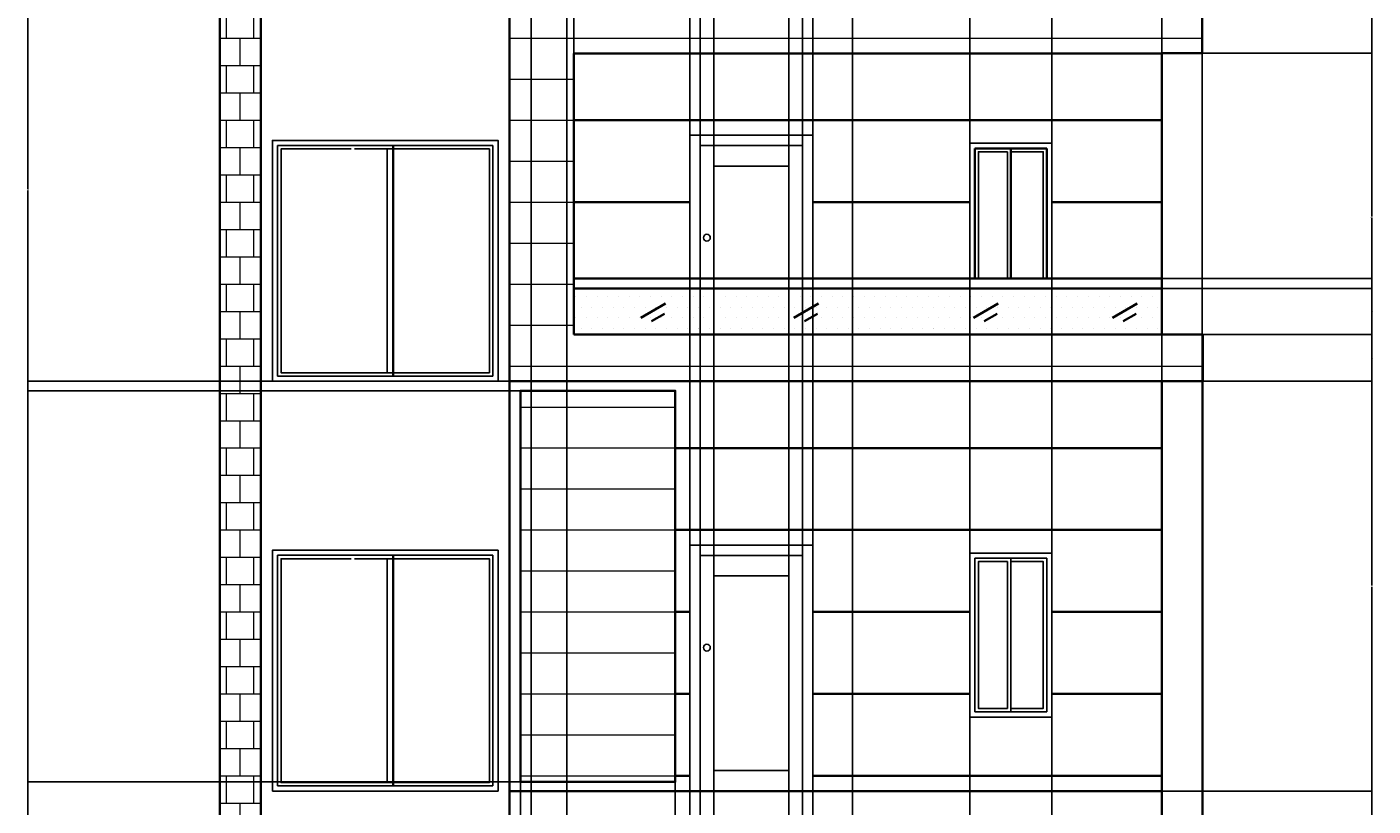
# Model space of a CAD drawing. Units: inches. Extents: x 10 to 404, y -77 to 696.
# Tile 3 of 5: x 10 to 404, y 135 to 363. Entities that reach past the tile are written whole.
import ezdxf

# ---------------------------------------------------------------- set-up
doc = ezdxf.new("R2010")
doc.units = ezdxf.units.IN
doc.header["$MEASUREMENT"] = 0
for name, color, linetype, lineweight in [('A-ANNO-DIMS', 2, 'Continuous', 18), ('A-DOOR', 4, 'Continuous', 25), ('A-ELEV', 7, 'Continuous', 35), ('A-ELEV-PATT', 8, 'Continuous', 13), ('A-GLAZ', 4, 'Continuous', 25)]:
    doc.layers.add(name, color=color, linetype=linetype, lineweight=lineweight)
doc.styles.get("Standard").update_dxf_attribs({"font": 'arial.ttf'})
doc.dimstyles.get("Standard").update_dxf_attribs({"dimtxt": 0.18, "dimasz": 0.18, "dimexe": 0.18, "dimexo": 0.0625, "dimgap": 0.09, "dimtad": 0, "dimtih": 1, "dimtoh": 1, "dimdec": 4, "dimzin": 0, "dimdsep": 46, "dimtxsty": 'Standard', "dimcen": 0.09, "dimadec": 0, "dimazin": 0, "dimtfac": 1, "dimtdec": 4, "dimtofl": 0, "dimtmove": 0, "dimatfit": 3, "dimfxl": 1, "dimtolj": 1, "dimtzin": 0, "dimarcsym": 0})

# ---------------------------------------------------------------- blocks, each defined once
blk = doc.blocks.new('*U5')
for p, q in [((1.5, 1.5), (1.5, 46.5)), ((1.5, 46.5), (12, 46.5)), ((12, 1.5), (12, 46.5)), ((12, 46.5), (22.5, 46.5)), ((22.5, 46.5), (22.5, 1.5)), ((12, 1.5), (1.5, 1.5)), ((22.5, 1.5), (12, 1.5))]:
    blk.add_line(p, q)
blk.add_lwpolyline([(0, 0), (0, 48), (24, 48), (24, 0)], close=True)
for points in [[(11, 45.5), (11, 2.5), (2.5, 2.5), (2.5, 45.5), (11, 45.5)], [(12, 45.5), (21.5, 45.5), (21.5, 2.5), (12, 2.5)]]:
    blk.add_lwpolyline(points)
blk = doc.blocks.new('*U4')
blk.add_lwpolyline([(3.12, 0.01), (0.12, 0.01), (0.12, 72.01), (36.12, 72.01), (36.12, 0.01), (33.12, 0.01)])
for points in [[(33.12, 68.99), (33.12, 0.01), (3.12, 0.01), (3.12, 68.99)], [(29.12, 6.01), (29.12, 62.99), (7.12, 62.99), (7.12, 6.01)]]:
    blk.add_lwpolyline(points, close=True)
blk.add_circle((31.12, 42.01), 1)
blk = doc.blocks.new('WIN-SLIDING-2P')
for p, q in [((83.01, 21.05), (83.01, 88.58)), ((83.01, 88.58), (105.51, 88.58)), ((105.51, 88.58), (146.03, 88.58)), ((146.03, 88.58), (146.03, 21.05)), ((105.51, 21.05), (83.01, 21.05)), ((146.03, 21.05), (105.51, 21.05))]:
    blk.add_line(p, q)
blk.add_lwpolyline([(81.51, 19.55), (81.51, 90.08), (147.53, 90.08), (147.53, 19.55)], close=True)
blk.add_lwpolyline([(115.07, 87.58), (115.07, 22.05), (84.01, 22.05), (84.01, 87.58), (104.51, 87.58)])
blk = doc.blocks.new('*D10')
at = {"layer": 'A-ANNO-DIMS', "color": 0, "lineweight": -2, "transparency": 16777216}
for p, q in [((65.94, 657.96), (9.76, 657.96)), ((9.94, 657.78), (9.94, 315.77)), ((9.94, -26.6), (9.94, 315.41)), ((176.46, -26.78), (9.76, -26.78))]:
    blk.add_line(p, q, dxfattribs=at)
at = {"layer": 'A-ANNO-DIMS', "color": 0, "transparency": 16777216}
for points in [[(9.91, 657.78), (9.97, 657.78), (9.94, 657.96)], [(9.91, -26.6), (9.97, -26.6), (9.94, -26.78)]]:
    blk.add_solid(points, dxfattribs=at)
at = {"layer": 'Defpoints', "color": 0, "transparency": 16777216}
for p in [(9.94, 657.96), (66.01, 657.96), (176.53, -26.78)]:
    blk.add_point(p, dxfattribs=at)
at = {"layer": 'A-ANNO-DIMS', "color": 0, "transparency": 16777216, "insert": (9.94, 315.59), "char_height": 0.18, "attachment_point": 5}
blk.add_mtext('\\A1;684.7', dxfattribs=at)
blk = doc.blocks.new('*D23')
at = {"layer": 'A-ANNO-DIMS', "color": 0, "lineweight": -2, "transparency": 16777216}
for p, q in [((341.87, 355.52), (341.87, -64.31)), ((353.59, 355.52), (353.59, -64.31)), ((342.05, -64.13), (347.27, -64.13)), ((353.41, -64.13), (348.18, -64.13))]:
    blk.add_line(p, q, dxfattribs=at)
at = {"layer": 'A-ANNO-DIMS', "color": 0, "transparency": 16777216}
for points in [[(342.05, -64.1), (342.05, -64.16), (341.87, -64.13)], [(353.41, -64.1), (353.41, -64.16), (353.59, -64.13)]]:
    blk.add_solid(points, dxfattribs=at)
at = {"layer": 'Defpoints', "color": 0, "transparency": 16777216}
for p in [(341.87, 355.58), (353.59, 355.58), (353.59, -64.13)]:
    blk.add_point(p, dxfattribs=at)
at = {"layer": 'A-ANNO-DIMS', "color": 0, "transparency": 16777216, "insert": (347.73, -64.13), "char_height": 0.18, "attachment_point": 5}
blk.add_mtext('\\A1;11.723', dxfattribs=at)
blk = doc.blocks.new('*D28')
at = {"layer": 'A-ANNO-DIMS', "color": 0, "lineweight": -2, "transparency": 16777216}
for p, q in [((341.93, 139.55), (403.47, 139.55)), ((403.29, 139.37), (403.29, 79.74)), ((403.29, 19.73), (403.29, 79.37)), ((341.93, 19.55), (403.47, 19.55))]:
    blk.add_line(p, q, dxfattribs=at)
at = {"layer": 'A-ANNO-DIMS', "color": 0, "transparency": 16777216}
for points in [[(403.26, 139.37), (403.32, 139.37), (403.29, 139.55)], [(403.26, 19.73), (403.32, 19.73), (403.29, 19.55)]]:
    blk.add_solid(points, dxfattribs=at)
at = {"layer": 'Defpoints', "color": 0, "transparency": 16777216}
for p in [(341.87, 139.55), (403.29, 139.55), (341.87, 19.55)]:
    blk.add_point(p, dxfattribs=at)
at = {"layer": 'A-ANNO-DIMS', "color": 0, "transparency": 16777216, "insert": (403.29, 79.55), "char_height": 0.18, "attachment_point": 5}
blk.add_mtext('\\A1;120', dxfattribs=at)
blk = doc.blocks.new('*D29')
at = {"layer": 'A-ANNO-DIMS', "color": 0, "lineweight": -2, "transparency": 16777216}
for p, q in [((341.93, 259.55), (403.47, 259.55)), ((403.29, 259.37), (403.29, 199.74)), ((403.29, 139.73), (403.29, 199.37)), ((341.93, 139.55), (403.47, 139.55))]:
    blk.add_line(p, q, dxfattribs=at)
at = {"layer": 'A-ANNO-DIMS', "color": 0, "transparency": 16777216}
for points in [[(403.26, 259.37), (403.32, 259.37), (403.29, 259.55)], [(403.26, 139.73), (403.32, 139.73), (403.29, 139.55)]]:
    blk.add_solid(points, dxfattribs=at)
at = {"layer": 'Defpoints', "color": 0, "transparency": 16777216}
for p in [(341.87, 259.55), (403.29, 259.55), (341.87, 139.55)]:
    blk.add_point(p, dxfattribs=at)
at = {"layer": 'A-ANNO-DIMS', "color": 0, "transparency": 16777216, "insert": (403.29, 199.55), "char_height": 0.18, "attachment_point": 5}
blk.add_mtext('\\A1;120', dxfattribs=at)
blk = doc.blocks.new('*D30')
at = {"layer": 'A-ANNO-DIMS', "color": 0, "lineweight": -2, "transparency": 16777216}
for p, q in [((353.65, 355.58), (403.47, 355.58)), ((403.29, 355.4), (403.29, 307.75)), ((403.29, 259.73), (403.29, 307.38)), ((341.93, 259.55), (403.47, 259.55))]:
    blk.add_line(p, q, dxfattribs=at)
at = {"layer": 'A-ANNO-DIMS', "color": 0, "transparency": 16777216}
for points in [[(403.26, 355.4), (403.32, 355.4), (403.29, 355.58)], [(403.26, 259.73), (403.32, 259.73), (403.29, 259.55)]]:
    blk.add_solid(points, dxfattribs=at)
at = {"layer": 'Defpoints', "color": 0, "transparency": 16777216}
for p in [(353.59, 355.58), (403.29, 355.58), (341.87, 259.55)]:
    blk.add_point(p, dxfattribs=at)
at = {"layer": 'A-ANNO-DIMS', "color": 0, "transparency": 16777216, "insert": (403.29, 307.57), "char_height": 0.18, "attachment_point": 5}
blk.add_mtext('\\A1;96.02', dxfattribs=at)
blk = doc.blocks.new('*D31')
at = {"layer": 'A-ANNO-DIMS', "color": 0, "lineweight": -2, "transparency": 16777216}
for p, q in [((353.65, 379.55), (403.47, 379.55)), ((403.29, 379.37), (403.29, 367.75)), ((403.29, 355.76), (403.29, 367.38)), ((353.65, 355.58), (403.47, 355.58))]:
    blk.add_line(p, q, dxfattribs=at)
at = {"layer": 'A-ANNO-DIMS', "color": 0, "transparency": 16777216}
for points in [[(403.26, 379.37), (403.32, 379.37), (403.29, 379.55)], [(403.26, 355.76), (403.32, 355.76), (403.29, 355.58)]]:
    blk.add_solid(points, dxfattribs=at)
at = {"layer": 'Defpoints', "color": 0, "transparency": 16777216}
for p in [(353.59, 379.55), (403.29, 379.55), (353.59, 355.58)]:
    blk.add_point(p, dxfattribs=at)
at = {"layer": 'A-ANNO-DIMS', "color": 0, "transparency": 16777216, "insert": (403.29, 367.57), "char_height": 0.18, "attachment_point": 5}
blk.add_mtext('\\A1;23.975', dxfattribs=at)
blk = doc.blocks.new('*D36')
at = {"layer": 'A-ANNO-DIMS', "color": 0, "lineweight": -2, "transparency": 16777216}
for p, q in [((353.93, 273.2), (403.47, 273.2)), ((403.29, 273.02), (403.29, 266.56)), ((403.29, 259.73), (403.29, 266.19)), ((353.93, 259.55), (403.47, 259.55))]:
    blk.add_line(p, q, dxfattribs=at)
at = {"layer": 'A-ANNO-DIMS', "color": 0, "transparency": 16777216}
for points in [[(403.26, 273.02), (403.32, 273.02), (403.29, 273.2)], [(403.26, 259.73), (403.32, 259.73), (403.29, 259.55)]]:
    blk.add_solid(points, dxfattribs=at)
at = {"layer": 'Defpoints', "color": 0, "transparency": 16777216}
for p in [(353.87, 273.2), (403.29, 273.2), (353.87, 259.55)]:
    blk.add_point(p, dxfattribs=at)
at = {"layer": 'A-ANNO-DIMS', "color": 0, "transparency": 16777216, "insert": (403.29, 266.38), "char_height": 0.18, "attachment_point": 5}
blk.add_mtext('\\A1;13.646', dxfattribs=at)
blk = doc.blocks.new('*D37')
at = {"layer": 'A-ANNO-DIMS', "color": 0, "lineweight": -2, "transparency": 16777216}
for p, q in [((341.93, 286.67), (403.47, 286.67)), ((403.29, 286.49), (403.29, 280.11)), ((403.29, 273.38), (403.29, 279.75)), ((341.93, 273.2), (403.47, 273.2))]:
    blk.add_line(p, q, dxfattribs=at)
at = {"layer": 'A-ANNO-DIMS', "color": 0, "transparency": 16777216}
for points in [[(403.26, 286.49), (403.32, 286.49), (403.29, 286.67)], [(403.26, 273.38), (403.32, 273.38), (403.29, 273.2)]]:
    blk.add_solid(points, dxfattribs=at)
at = {"layer": 'Defpoints', "color": 0, "transparency": 16777216}
for p in [(341.87, 286.67), (403.29, 286.67), (341.87, 273.2)]:
    blk.add_point(p, dxfattribs=at)
at = {"layer": 'A-ANNO-DIMS', "color": 0, "transparency": 16777216, "insert": (403.29, 279.93), "char_height": 0.18, "attachment_point": 5}
blk.add_mtext('\\A1;13.467', dxfattribs=at)
blk = doc.blocks.new('*D38')
at = {"layer": 'A-ANNO-DIMS', "color": 0, "lineweight": -2, "transparency": 16777216}
for p, q in [((341.93, 289.59), (403.47, 289.59)), ((403.29, 289.41), (403.29, 288.31)), ((403.29, 286.85), (403.29, 287.95)), ((341.93, 286.67), (403.47, 286.67))]:
    blk.add_line(p, q, dxfattribs=at)
at = {"layer": 'A-ANNO-DIMS', "color": 0, "transparency": 16777216}
for points in [[(403.26, 289.41), (403.32, 289.41), (403.29, 289.59)], [(403.26, 286.85), (403.32, 286.85), (403.29, 286.67)]]:
    blk.add_solid(points, dxfattribs=at)
at = {"layer": 'Defpoints', "color": 0, "transparency": 16777216}
for p in [(341.87, 289.59), (403.29, 289.59), (341.87, 286.67)]:
    blk.add_point(p, dxfattribs=at)
at = {"layer": 'A-ANNO-DIMS', "color": 0, "transparency": 16777216, "insert": (403.29, 288.13), "char_height": 0.18, "attachment_point": 5}
blk.add_mtext('\\A1;2.92', dxfattribs=at)
blk = doc.blocks.new('*D39')
at = {"layer": 'A-ANNO-DIMS', "color": 0, "lineweight": -2, "transparency": 16777216}
for p, q in [((341.87, 259.49), (341.87, -64.31)), ((353.87, 259.49), (353.87, -64.31)), ((342.05, -64.13), (347.66, -64.13)), ((353.69, -64.13), (348.08, -64.13))]:
    blk.add_line(p, q, dxfattribs=at)
at = {"layer": 'A-ANNO-DIMS', "color": 0, "transparency": 16777216}
for points in [[(342.05, -64.1), (342.05, -64.16), (341.87, -64.13)], [(353.69, -64.1), (353.69, -64.16), (353.87, -64.13)]]:
    blk.add_solid(points, dxfattribs=at)
at = {"layer": 'Defpoints', "color": 0, "transparency": 16777216}
for p in [(341.87, 259.55), (353.87, 259.55), (353.87, -64.13)]:
    blk.add_point(p, dxfattribs=at)
at = {"layer": 'A-ANNO-DIMS', "color": 0, "transparency": 16777216, "insert": (347.87, -64.13), "char_height": 0.18, "attachment_point": 5}
blk.add_mtext('\\A1;12', dxfattribs=at)
blk = doc.blocks.new('*D40')
at = {"layer": 'A-ANNO-DIMS', "color": 0, "lineweight": -2, "transparency": 16777216}
for p, q in [((150.93, 259.62), (150.93, 695.87)), ((151.11, 695.69), (159.89, 695.69)), ((169.58, 695.69), (160.8, 695.69)), ((169.76, 289.65), (169.76, 695.87))]:
    blk.add_line(p, q, dxfattribs=at)
at = {"layer": 'A-ANNO-DIMS', "color": 0, "transparency": 16777216}
for points in [[(151.11, 695.72), (151.11, 695.66), (150.93, 695.69)], [(169.58, 695.72), (169.58, 695.66), (169.76, 695.69)]]:
    blk.add_solid(points, dxfattribs=at)
at = {"layer": 'Defpoints', "color": 0, "transparency": 16777216}
for p in [(169.76, 695.69), (169.76, 289.59), (150.93, 259.55)]:
    blk.add_point(p, dxfattribs=at)
at = {"layer": 'A-ANNO-DIMS', "color": 0, "transparency": 16777216, "insert": (160.35, 695.69), "char_height": 0.18, "attachment_point": 5}
blk.add_mtext('\\A1;18.827', dxfattribs=at)
blk = doc.blocks.new('*D41')
at = {"layer": 'A-ANNO-DIMS', "color": 0, "lineweight": -2, "transparency": 16777216}
for p, q in [((169.76, 289.65), (169.76, 695.87)), ((169.94, 695.69), (255.45, 695.69)), ((341.69, 695.69), (256.18, 695.69)), ((341.87, 289.65), (341.87, 695.87))]:
    blk.add_line(p, q, dxfattribs=at)
at = {"layer": 'A-ANNO-DIMS', "color": 0, "transparency": 16777216}
for points in [[(169.94, 695.72), (169.94, 695.66), (169.76, 695.69)], [(341.69, 695.72), (341.69, 695.66), (341.87, 695.69)]]:
    blk.add_solid(points, dxfattribs=at)
at = {"layer": 'Defpoints', "color": 0, "transparency": 16777216}
for p in [(341.87, 695.69), (169.76, 289.59), (341.87, 289.59)]:
    blk.add_point(p, dxfattribs=at)
at = {"layer": 'A-ANNO-DIMS', "color": 0, "transparency": 16777216, "insert": (255.81, 695.69), "char_height": 0.18, "attachment_point": 5}
blk.add_mtext('\\A1;172.1', dxfattribs=at)
blk = doc.blocks.new('*D42')
at = {"layer": 'A-ANNO-DIMS', "color": 0, "lineweight": -2, "transparency": 16777216}
for p, q in [((150.93, 259.49), (150.93, -64.31)), ((154.06, 142.19), (154.06, -64.31)), ((151.11, -64.13), (152.17, -64.13)), ((153.88, -64.13), (152.82, -64.13))]:
    blk.add_line(p, q, dxfattribs=at)
at = {"layer": 'A-ANNO-DIMS', "color": 0, "transparency": 16777216}
for points in [[(151.11, -64.1), (151.11, -64.16), (150.93, -64.13)], [(153.88, -64.1), (153.88, -64.16), (154.06, -64.13)]]:
    blk.add_solid(points, dxfattribs=at)
at = {"layer": 'Defpoints', "color": 0, "transparency": 16777216}
for p in [(150.93, 259.55), (154.06, 142.25), (154.06, -64.13)]:
    blk.add_point(p, dxfattribs=at)
at = {"layer": 'A-ANNO-DIMS', "color": 0, "transparency": 16777216, "insert": (152.5, -64.13), "char_height": 0.18, "attachment_point": 5}
blk.add_mtext('\\A1;3.13', dxfattribs=at)
blk = doc.blocks.new('*D43')
at = {"layer": 'A-ANNO-DIMS', "color": 0, "lineweight": -2, "transparency": 16777216}
for p, q in [((154.06, 142.19), (154.06, -64.31)), ((199.39, 142.19), (199.39, -64.31)), ((154.24, -64.13), (176.33, -64.13)), ((199.21, -64.13), (177.13, -64.13))]:
    blk.add_line(p, q, dxfattribs=at)
at = {"layer": 'A-ANNO-DIMS', "color": 0, "transparency": 16777216}
for points in [[(154.24, -64.1), (154.24, -64.16), (154.06, -64.13)], [(199.21, -64.1), (199.21, -64.16), (199.39, -64.13)]]:
    blk.add_solid(points, dxfattribs=at)
at = {"layer": 'Defpoints', "color": 0, "transparency": 16777216}
for p in [(154.06, 142.25), (199.39, 142.25), (199.39, -64.13)]:
    blk.add_point(p, dxfattribs=at)
at = {"layer": 'A-ANNO-DIMS', "color": 0, "transparency": 16777216, "insert": (176.73, -64.13), "char_height": 0.18, "attachment_point": 5}
blk.add_mtext('\\A1;45.33', dxfattribs=at)
blk = doc.blocks.new('*D44')
at = {"layer": 'A-ANNO-DIMS', "color": 0, "lineweight": -2, "transparency": 16777216}
for p, q in [((154, 256.74), (9.76, 256.74)), ((9.94, 256.56), (9.94, 199.68)), ((9.94, 142.43), (9.94, 199.31)), ((154, 142.25), (9.76, 142.25))]:
    blk.add_line(p, q, dxfattribs=at)
at = {"layer": 'A-ANNO-DIMS', "color": 0, "transparency": 16777216}
for points in [[(9.91, 256.56), (9.97, 256.56), (9.94, 256.74)], [(9.91, 142.43), (9.97, 142.43), (9.94, 142.25)]]:
    blk.add_solid(points, dxfattribs=at)
at = {"layer": 'Defpoints', "color": 0, "transparency": 16777216}
for p in [(9.94, 256.74), (154.06, 256.74), (154.06, 142.25)]:
    blk.add_point(p, dxfattribs=at)
at = {"layer": 'A-ANNO-DIMS', "color": 0, "transparency": 16777216, "insert": (9.94, 199.5), "char_height": 0.18, "attachment_point": 5}
blk.add_mtext('\\A1;114.5', dxfattribs=at)
blk = doc.blocks.new('*D45')
at = {"layer": 'A-ANNO-DIMS', "color": 0, "lineweight": -2, "transparency": 16777216}
for p, q in [((150.87, 259.55), (9.76, 259.55)), ((154, 256.74), (9.76, 256.74)), ((9.94, 259.37), (9.94, 258.33)), ((9.94, 256.92), (9.94, 257.97))]:
    blk.add_line(p, q, dxfattribs=at)
at = {"layer": 'A-ANNO-DIMS', "color": 0, "transparency": 16777216}
for points in [[(9.91, 259.37), (9.97, 259.37), (9.94, 259.55)], [(9.91, 256.92), (9.97, 256.92), (9.94, 256.74)]]:
    blk.add_solid(points, dxfattribs=at)
at = {"layer": 'Defpoints', "color": 0, "transparency": 16777216}
for p in [(9.94, 259.55), (150.93, 259.55), (154.06, 256.74)]:
    blk.add_point(p, dxfattribs=at)
at = {"layer": 'A-ANNO-DIMS', "color": 0, "transparency": 16777216, "insert": (9.94, 258.15), "char_height": 0.18, "attachment_point": 5}
blk.add_mtext('\\A1;2.809', dxfattribs=at)
blk = doc.blocks.new('*D48')
at = {"layer": 'A-ANNO-DIMS', "color": 0, "lineweight": -2, "transparency": 16777216}
for p, q in [((285.62, 521.17), (285.62, -64.31)), ((239.67, 499.54), (239.67, -64.31)), ((239.85, -64.13), (262.25, -64.13)), ((285.44, -64.13), (263.04, -64.13))]:
    blk.add_line(p, q, dxfattribs=at)
at = {"layer": 'A-ANNO-DIMS', "color": 0, "transparency": 16777216}
for points in [[(239.85, -64.1), (239.85, -64.16), (239.67, -64.13)], [(285.44, -64.1), (285.44, -64.16), (285.62, -64.13)]]:
    blk.add_solid(points, dxfattribs=at)
at = {"layer": 'Defpoints', "color": 0, "transparency": 16777216}
for p in [(285.62, 521.23), (239.67, 499.6), (285.62, -64.13)]:
    blk.add_point(p, dxfattribs=at)
at = {"layer": 'A-ANNO-DIMS', "color": 0, "transparency": 16777216, "insert": (262.64, -64.13), "char_height": 0.18, "attachment_point": 5}
blk.add_mtext('\\A1;45.95', dxfattribs=at)
blk = doc.blocks.new('*D49')
at = {"layer": 'A-ANNO-DIMS', "color": 0, "lineweight": -2, "transparency": 16777216}
for p, q in [((285.62, 521.17), (285.62, -64.31)), ((309.62, 521.17), (309.62, -64.31)), ((285.8, -64.13), (297.4, -64.13)), ((309.44, -64.13), (297.84, -64.13))]:
    blk.add_line(p, q, dxfattribs=at)
at = {"layer": 'A-ANNO-DIMS', "color": 0, "transparency": 16777216}
for points in [[(285.8, -64.1), (285.8, -64.16), (285.62, -64.13)], [(309.44, -64.1), (309.44, -64.16), (309.62, -64.13)]]:
    blk.add_solid(points, dxfattribs=at)
at = {"layer": 'Defpoints', "color": 0, "transparency": 16777216}
for p in [(285.62, 521.23), (309.62, 521.23), (309.62, -64.13)]:
    blk.add_point(p, dxfattribs=at)
at = {"layer": 'A-ANNO-DIMS', "color": 0, "transparency": 16777216, "insert": (297.62, -64.13), "char_height": 0.18, "attachment_point": 5}
blk.add_mtext('\\A1;24', dxfattribs=at)
blk = doc.blocks.new('*D50')
at = {"layer": 'A-ANNO-DIMS', "color": 0, "lineweight": -2, "transparency": 16777216}
for p, q in [((157.2, 100.31), (157.2, 695.87)), ((157.38, 695.69), (161.98, 695.69)), ((167.49, 695.69), (162.89, 695.69)), ((167.67, 91.62), (167.67, 695.87))]:
    blk.add_line(p, q, dxfattribs=at)
at = {"layer": 'A-ANNO-DIMS', "color": 0, "transparency": 16777216}
for points in [[(157.38, 695.72), (157.38, 695.66), (157.2, 695.69)], [(167.49, 695.72), (167.49, 695.66), (167.67, 695.69)]]:
    blk.add_solid(points, dxfattribs=at)
at = {"layer": 'Defpoints', "color": 0, "transparency": 16777216}
for p in [(167.67, 695.69), (157.2, 100.24), (167.67, 91.55)]:
    blk.add_point(p, dxfattribs=at)
at = {"layer": 'A-ANNO-DIMS', "color": 0, "transparency": 16777216, "insert": (162.43, 695.69), "char_height": 0.18, "attachment_point": 5}
blk.add_mtext('\\A1;10.469', dxfattribs=at)
blk = doc.blocks.new('*D51')
at = {"layer": 'A-ANNO-DIMS', "color": 0, "lineweight": -2, "transparency": 16777216}
for p, q in [((167.67, 91.62), (167.67, 695.87)), ((167.85, 695.69), (209.06, 695.69)), ((251.06, 695.69), (209.85, 695.69)), ((251.24, 100.31), (251.24, 695.87))]:
    blk.add_line(p, q, dxfattribs=at)
at = {"layer": 'A-ANNO-DIMS', "color": 0, "transparency": 16777216}
for points in [[(167.85, 695.72), (167.85, 695.66), (167.67, 695.69)], [(251.06, 695.72), (251.06, 695.66), (251.24, 695.69)]]:
    blk.add_solid(points, dxfattribs=at)
at = {"layer": 'Defpoints', "color": 0, "transparency": 16777216}
for p in [(251.24, 695.69), (251.24, 100.24), (167.67, 91.55)]:
    blk.add_point(p, dxfattribs=at)
at = {"layer": 'A-ANNO-DIMS', "color": 0, "transparency": 16777216, "insert": (209.45, 695.69), "char_height": 0.18, "attachment_point": 5}
blk.add_mtext('\\A1;83.57', dxfattribs=at)
blk = doc.blocks.new('*D61')
at = {"layer": 'A-ANNO-DIMS', "color": 0, "lineweight": -2, "transparency": 16777216}
for p, q in [((206.67, 19.62), (206.67, 695.87)), ((206.85, 695.69), (208.51, 695.69)), ((210.49, 695.69), (208.82, 695.69)), ((210.67, 25.62), (210.67, 695.87))]:
    blk.add_line(p, q, dxfattribs=at)
at = {"layer": 'A-ANNO-DIMS', "color": 0, "transparency": 16777216}
for points in [[(206.85, 695.72), (206.85, 695.66), (206.67, 695.69)], [(210.49, 695.72), (210.49, 695.66), (210.67, 695.69)]]:
    blk.add_solid(points, dxfattribs=at)
at = {"layer": 'Defpoints', "color": 0, "transparency": 16777216}
for p in [(210.67, 695.69), (210.67, 25.55), (206.67, 19.55)]:
    blk.add_point(p, dxfattribs=at)
at = {"layer": 'A-ANNO-DIMS', "color": 0, "transparency": 16777216, "insert": (208.67, 695.69), "char_height": 0.18, "attachment_point": 5}
blk.add_mtext('\\A1;4', dxfattribs=at)
blk = doc.blocks.new('*D62')
at = {"layer": 'A-ANNO-DIMS', "color": 0, "lineweight": -2, "transparency": 16777216}
for p, q in [((210.67, 25.62), (210.67, 695.87)), ((210.85, 695.69), (221.45, 695.69)), ((232.49, 695.69), (221.89, 695.69)), ((232.67, 25.62), (232.67, 695.87))]:
    blk.add_line(p, q, dxfattribs=at)
at = {"layer": 'A-ANNO-DIMS', "color": 0, "transparency": 16777216}
for points in [[(210.85, 695.72), (210.85, 695.66), (210.67, 695.69)], [(232.49, 695.72), (232.49, 695.66), (232.67, 695.69)]]:
    blk.add_solid(points, dxfattribs=at)
at = {"layer": 'Defpoints', "color": 0, "transparency": 16777216}
for p in [(232.67, 695.69), (210.67, 25.55), (232.67, 25.55)]:
    blk.add_point(p, dxfattribs=at)
at = {"layer": 'A-ANNO-DIMS', "color": 0, "transparency": 16777216, "insert": (221.67, 695.69), "char_height": 0.18, "attachment_point": 5}
blk.add_mtext('\\A1;22', dxfattribs=at)
blk = doc.blocks.new('*D66')
at = {"layer": 'A-ANNO-DIMS', "color": 0, "lineweight": -2, "transparency": 16777216}
for p, q in [((203.67, 499.54), (203.67, -64.31)), ((206.67, 499.54), (206.67, -64.31)), ((203.85, -64.13), (205.02, -64.13)), ((206.49, -64.13), (205.32, -64.13))]:
    blk.add_line(p, q, dxfattribs=at)
at = {"layer": 'A-ANNO-DIMS', "color": 0, "transparency": 16777216}
for points in [[(203.85, -64.1), (203.85, -64.16), (203.67, -64.13)], [(206.49, -64.1), (206.49, -64.16), (206.67, -64.13)]]:
    blk.add_solid(points, dxfattribs=at)
at = {"layer": 'Defpoints', "color": 0, "transparency": 16777216}
for p in [(203.67, 499.6), (206.67, 499.6), (206.67, -64.13)]:
    blk.add_point(p, dxfattribs=at)
at = {"layer": 'A-ANNO-DIMS', "color": 0, "transparency": 16777216, "insert": (205.17, -64.13), "char_height": 0.18, "attachment_point": 5}
blk.add_mtext('\\A1;3', dxfattribs=at)
blk = doc.blocks.new('*D67')
at = {"layer": 'A-ANNO-DIMS', "color": 0, "lineweight": -2, "transparency": 16777216}
for p, q in [((206.67, 499.54), (206.67, -64.31)), ((236.67, 499.54), (236.67, -64.31)), ((206.85, -64.13), (221.45, -64.13)), ((236.49, -64.13), (221.89, -64.13))]:
    blk.add_line(p, q, dxfattribs=at)
at = {"layer": 'A-ANNO-DIMS', "color": 0, "transparency": 16777216}
for points in [[(206.85, -64.1), (206.85, -64.16), (206.67, -64.13)], [(236.49, -64.1), (236.49, -64.16), (236.67, -64.13)]]:
    blk.add_solid(points, dxfattribs=at)
at = {"layer": 'Defpoints', "color": 0, "transparency": 16777216}
for p in [(206.67, 499.6), (236.67, 499.6), (236.67, -64.13)]:
    blk.add_point(p, dxfattribs=at)
at = {"layer": 'A-ANNO-DIMS', "color": 0, "transparency": 16777216, "insert": (221.67, -64.13), "char_height": 0.18, "attachment_point": 5}
blk.add_mtext('\\A1;30', dxfattribs=at)
blk = doc.blocks.new('*D68')
at = {"layer": 'A-ANNO-DIMS', "color": 0, "lineweight": -2, "transparency": 16777216}
for p, q in [((236.67, 499.54), (236.67, -64.31)), ((239.67, 499.54), (239.67, -64.31)), ((236.85, -64.13), (238.02, -64.13)), ((239.49, -64.13), (238.32, -64.13))]:
    blk.add_line(p, q, dxfattribs=at)
at = {"layer": 'A-ANNO-DIMS', "color": 0, "transparency": 16777216}
for points in [[(236.85, -64.1), (236.85, -64.16), (236.67, -64.13)], [(239.49, -64.1), (239.49, -64.16), (239.67, -64.13)]]:
    blk.add_solid(points, dxfattribs=at)
at = {"layer": 'Defpoints', "color": 0, "transparency": 16777216}
for p in [(236.67, 499.6), (239.67, 499.6), (239.67, -64.13)]:
    blk.add_point(p, dxfattribs=at)
at = {"layer": 'A-ANNO-DIMS', "color": 0, "transparency": 16777216, "insert": (238.17, -64.13), "char_height": 0.18, "attachment_point": 5}
blk.add_mtext('\\A1;3', dxfattribs=at)

msp = doc.modelspace()

# ---------------------------------------------------------------- hatches: boundary and pattern name
at = {"layer": 'A-ELEV-PATT'}
h = msp.add_hatch(dxfattribs=at)
h.set_pattern_fill('_USER', color=256, scale=12, pattern_type=0)
h.set_pattern_definition([(0, (0, 0), (0, 12), [])])
h.paths.add_polyline_path([(188.1159, 499.5535), (150.9344, 499.5535), (150.9344, 379.5535), (188.1159, 379.5535)])
h.paths.add_polyline_path([(188.1159, 585.1332), (354.5631, 585.1332), (354.5631, 619.5535), (341.8668, 619.5535), (150.9344, 619.5535), (150.9344, 499.5535), (188.1159, 499.5535)])
h.paths.add_polyline_path([(353.5898, 379.5535), (341.8668, 379.5535), (150.9344, 379.5535), (150.9344, 259.5535), (341.8668, 259.5535), (353.8668, 259.5535), (353.8668, 273.1993), (341.8668, 273.1993), (169.7618, 273.1993), (169.7618, 355.5535), (341.8668, 355.5535), (341.8668, 355.5783), (353.5898, 355.5783)])
h.paths.add_polyline_path([(285.6197, 451.5918), (239.6671, 451.5918), (239.6671, 379.5535), (309.6197, 379.5535), (309.6197, 403.5918), (285.6197, 403.5918)])
h.paths.add_polyline_path([(199.3943, 256.7444), (154.0619, 256.7444), (154.0619, 142.2479), (199.3943, 142.2479)])
h = msp.add_hatch(dxfattribs=at)
h.set_pattern_fill('_USER', color=256, scale=24, pattern_type=0)
h.set_pattern_definition([(0, (0, 0), (0, 24), [])])
h.paths.add_polyline_path([(341.8668, 139.5535), (150.9344, 139.5535), (150.9344, 19.5535), (167.6671, 19.5535), (167.6671, 91.5535), (157.1984, 91.5535), (157.1984, 100.244), (251.2392, 100.244), (251.2392, 91.5535), (239.6671, 91.5535), (239.6671, 19.5535), (341.8668, 19.5535)])
h.paths.add_polyline_path([(285.6197, 89.2337), (309.6197, 89.2337), (309.6197, 41.2337), (285.6197, 41.2337)], flags=16)
h.paths.add_polyline_path([(287.1197, 87.7337), (297.6197, 87.7337), (308.1197, 87.7337), (308.1197, 42.7337), (297.6197, 42.7337), (287.1197, 42.7337)], flags=0)
h.paths.add_polyline_path([(288.1197, 86.7337), (296.6197, 86.7337), (296.6197, 43.7337), (288.1197, 43.7337)], flags=0)
h.paths.add_polyline_path([(297.6197, 86.7337), (307.1197, 86.7337), (307.1197, 43.7337), (297.6197, 43.7337)], flags=0)
h.paths.add_polyline_path([(341.8668, 585.1332), (188.1159, 585.1332), (188.1159, 499.5535), (203.6671, 499.5535), (203.6671, 571.6046), (239.6671, 571.6046), (239.6671, 499.5535), (341.8668, 499.5535)])
h.paths.add_polyline_path([(285.6197, 521.2337), (285.6197, 569.2337), (309.6197, 569.2337), (309.6197, 521.2337)], flags=16)
h.paths.add_polyline_path([(287.1197, 522.7337), (287.1197, 567.7337), (297.6197, 567.7337), (308.1197, 567.7337), (308.1197, 522.7337), (297.6197, 522.7337)], flags=0)
h.paths.add_polyline_path([(288.1197, 523.7337), (288.1197, 566.7337), (296.6197, 566.7337), (296.6197, 523.7337)], flags=0)
h.paths.add_polyline_path([(297.6197, 566.7337), (307.1197, 566.7337), (307.1197, 523.7337), (297.6197, 523.7337)], flags=0)
h = msp.add_hatch(dxfattribs=at)
h.set_pattern_fill('AR-B88', color=256)
h.paths.add_polyline_path([(78.1013, 499.5535), (66.1013, 499.5535), (66.1013, 19.5535), (78.1013, 19.5535)])
h = msp.add_hatch(dxfattribs=at)
h.set_pattern_fill('DOTS', color=256, scale=1100)
h.paths.add_polyline_path([(341.8668, 286.6666), (169.7618, 286.6666), (169.7618, 273.1993), (341.8668, 273.1993)])
h = msp.add_hatch(dxfattribs=at)
h.set_pattern_fill('DOTS', color=256, scale=50)
h.paths.add_polyline_path([(341.8668, 286.6666), (169.7618, 286.6666), (169.7618, 273.1993), (341.8668, 273.1993)])

# ---------------------------------------------------------------- linework, layer by layer
at = {"layer": 'A-DOOR'}
for points in [[(239.6671, 289.5881), (239.6671, 331.5791), (203.6671, 331.5791), (203.6671, 289.5881)], [(236.6671, 289.5881), (236.6671, 328.5561), (206.6671, 328.5561), (206.6671, 289.5881)], [(210.6671, 289.5881), (210.6671, 322.5561), (232.6671, 322.5561), (232.6671, 289.5881)], [(203.6671, 259.5791), (206.6671, 259.5791)], [(206.6671, 259.5791), (236.6671, 259.5791)], [(236.6671, 259.5791), (239.6671, 259.5791)]]:
    msp.add_lwpolyline(points, dxfattribs=at)
msp.add_circle((208.6671, 301.5791), 1, dxfattribs=at)
at = {"layer": 'A-ELEV'}
for p, q in [((66.1013, 619.5535), (66.1013, 19.5535)), ((78.1013, 619.5535), (78.1013, 19.5535)), ((150.9344, 19.5535), (150.9344, 619.5535)), ((341.8668, 355.5535), (169.7618, 355.5535)), ((169.7618, 355.5535), (169.7618, 273.1993)), ((341.8668, 273.1993), (341.8668, 355.5783)), ((341.8668, 355.5783), (341.8668, 355.5535)), ((169.7618, 336), (341.8668, 336)), ((116.8527, 261.0535), (116.8527, 328.5811)), ((287.1197, 327.7337), (297.6197, 327.7337)), ((287.1197, 289.5881), (287.1197, 327.7337)), ((297.6197, 327.7337), (308.1197, 327.7337)), ((297.6197, 289.5881), (297.6197, 327.7337)), ((308.1197, 327.7337), (308.1197, 289.5881)), ((169.7618, 312), (203.6671, 312)), ((239.6671, 312), (285.6197, 312)), ((309.6197, 312), (341.8668, 312)), ((189.3304, 278.1617), (196.5841, 282.3496)), ((234.1119, 278.1617), (241.3656, 282.3496)), ((286.6542, 278.1617), (293.9079, 282.3496)), ((327.3985, 278.1617), (334.6522, 282.3496)), ((192.4856, 277.1529), (196.2692, 279.3374)), ((237.2671, 277.1529), (241.0507, 279.3374)), ((289.8093, 277.1529), (293.593, 279.3374)), ((330.5536, 277.1529), (334.3373, 279.3374)), ((169.7618, 273.1993), (341.8668, 273.1993)), ((341.8668, 259.5535), (150.9344, 259.5535)), ((150.9344, 259.5535), (341.8668, 259.5535)), ((341.8668, 139.5535), (341.8668, 259.5535)), ((199.3943, 240), (341.8668, 240)), ((199.3943, 216), (341.8668, 216)), ((116.8527, 141.0535), (116.8527, 208.5811)), ((199.3943, 192), (203.6671, 192)), ((239.6671, 192), (285.6197, 192)), ((309.6197, 192), (341.8668, 192)), ((199.3943, 168), (203.6671, 168)), ((239.6671, 168), (285.6197, 168)), ((309.6197, 168), (341.8668, 168)), ((199.3943, 144), (203.6671, 144)), ((239.6671, 144), (341.8668, 144)), ((341.8668, 139.5535), (150.9344, 139.5535)), ((150.9344, 139.5535), (341.8668, 139.5535)), ((341.8668, 19.5535), (341.8668, 139.5535))]:
    msp.add_line(p, q, dxfattribs=at)
for points in [[(341.8668, 379.5535), (353.5898, 379.5535), (353.5898, 355.5783), (341.8668, 355.5783)], [(341.8668, 273.1993), (353.8668, 273.1993), (353.8668, 259.5535), (341.8668, 259.5535)]]:
    msp.add_lwpolyline(points, dxfattribs=at)
for points in [[(169.7618, 289.5881), (341.8668, 289.5881), (341.8668, 286.6666), (169.7618, 286.6666)], [(154.0619, 142.2479), (199.3943, 142.2479), (199.3943, 256.7444), (154.0619, 256.7444)]]:
    msp.add_lwpolyline(points, close=True, dxfattribs=at)
at = {"layer": 'A-GLAZ'}
for points in [[(105.5054, 327.5811), (145.0304, 327.5811), (145.0304, 262.0535), (105.5054, 262.0535)], [(285.6197, 289.5881), (285.6197, 329.2337), (309.6197, 329.2337), (309.6197, 289.5881)], [(288.1197, 289.5881), (288.1197, 326.7337), (296.6197, 326.7337)], [(296.6197, 326.7338), (296.6197, 289.5881)], [(297.6197, 326.7337), (307.1197, 326.7337), (307.1197, 289.5881)], [(105.5054, 207.5811), (145.0304, 207.5811), (145.0304, 142.0535), (105.5054, 142.0535)]]:
    msp.add_lwpolyline(points, dxfattribs=at)

# ---------------------------------------------------------------- block references
at = {"layer": 'A-DOOR', "xscale": -1}
msp.add_blockref('*U4', (239.7909, 139.5535), dxfattribs=at)
at = {"layer": 'A-GLAZ'}
for name, p in [('WIN-SLIDING-2P', (0, 240)), ('WIN-SLIDING-2P', (0, 120)), ('*U5', (285.6197, 161.2337))]:
    msp.add_blockref(name, p, dxfattribs=at)

# ---------------------------------------------------------------- dimensions: what is measured, and where the dimension line sits
at = {"layer": 'A-ANNO-DIMS'}
for base, p1, p2, override, picture, middle in [((169.7618, 695.6911), (150.9344, 259.5535), (169.7618, 289.5881), {"dimdec": 3, "dimlfac": 1, "dimrnd": 0, "dimzin": 0, "dimdsep": 46, "dimlunit": 2}, '*D40', (160.3481, 695.6911)), ((167.6671, 695.6911), (157.1984, 100.244), (167.6671, 91.5535), {"dimdec": 3, "dimlfac": 1, "dimrnd": 0, "dimzin": 0, "dimdsep": 46, "dimlunit": 2}, '*D50', (162.4328, 695.6911)), ((251.2392, 695.6911), (167.6671, 91.5535), (251.2392, 100.244), {"dimdec": 2, "dimlfac": 1, "dimrnd": 0, "dimzin": 0, "dimdsep": 46, "dimlunit": 2}, '*D51', (209.4531, 695.6911)), ((341.8668, 695.6911), (169.7618, 289.5881), (341.8668, 289.5881), {"dimdec": 1, "dimlfac": 1, "dimrnd": 0, "dimzin": 0, "dimdsep": 46, "dimlunit": 2}, '*D41', (255.8143, 695.6911)), ((210.6671, 695.6911), (206.6671, 19.5535), (210.6671, 25.5535), {"dimdec": 0, "dimlfac": 1, "dimrnd": 0, "dimzin": 0, "dimdsep": 46, "dimlunit": 2}, '*D61', (208.6671, 695.6911)), ((232.6671, 695.6911), (210.6671, 25.5535), (232.6671, 25.5535), {"dimdec": 0, "dimlfac": 1, "dimrnd": 0, "dimzin": 0, "dimdsep": 46, "dimlunit": 2}, '*D62', (221.6671, 695.6911)), ((285.6197, -64.1316), (239.6671, 499.6046), (285.6197, 521.2337), {"dimdec": 2, "dimlfac": 1, "dimrnd": 0, "dimzin": 0, "dimdsep": 46, "dimlunit": 2}, '*D48', (262.6434, -64.1316)), ((309.6197, -64.1316), (285.6197, 521.2337), (309.6197, 521.2337), {"dimdec": 0, "dimlfac": 1, "dimrnd": 0, "dimzin": 0, "dimdsep": 46, "dimlunit": 2}, '*D49', (297.6197, -64.1316)), ((206.6671, -64.1316), (203.6671, 499.6046), (206.6671, 499.6046), {"dimdec": 0, "dimlfac": 1, "dimrnd": 0, "dimzin": 0, "dimdsep": 46, "dimlunit": 2}, '*D66', (205.1671, -64.1316)), ((236.6671, -64.1316), (206.6671, 499.6046), (236.6671, 499.6046), {"dimdec": 0, "dimlfac": 1, "dimrnd": 0, "dimzin": 0, "dimdsep": 46, "dimlunit": 2}, '*D67', (221.6671, -64.1316)), ((239.6671, -64.1316), (236.6671, 499.6046), (239.6671, 499.6046), {"dimdec": 0, "dimlfac": 1, "dimrnd": 0, "dimzin": 0, "dimdsep": 46, "dimlunit": 2}, '*D68', (238.1671, -64.1316)), ((353.5898, -64.1316), (341.8668, 355.5783), (353.5898, 355.5783), {"dimdec": 3, "dimlfac": 1, "dimrnd": 0, "dimzin": 0, "dimdsep": 46, "dimlunit": 2}, '*D23', (347.7283, -64.1316)), ((154.0619, -64.1316), (150.9344, 259.5535), (154.0619, 142.2479), {"dimdec": 2, "dimlfac": 1, "dimrnd": 0, "dimzin": 0, "dimdsep": 46, "dimlunit": 2}, '*D42', (152.4982, -64.1316)), ((353.8668, -64.1316), (341.8668, 259.5535), (353.8668, 259.5535), {"dimdec": 0, "dimlfac": 1, "dimrnd": 0, "dimzin": 0, "dimdsep": 46, "dimlunit": 2}, '*D39', (347.8668, -64.1316)), ((199.3943, -64.1316), (154.0619, 142.2479), (199.3943, 142.2479), {"dimdec": 2, "dimlfac": 1, "dimrnd": 0, "dimzin": 0, "dimdsep": 46, "dimlunit": 2}, '*D43', (176.7281, -64.1316))]:
    dim = msp.add_linear_dim(base=base, p1=p1, p2=p2, dimstyle='Standard', override=override, dxfattribs=at)
    dim.commit()
    dim.dimension.update_dxf_attribs({"geometry": picture, "text_midpoint": middle})
for base, p1, p2, override, picture, middle in [((9.9405, 657.9612), (176.5266, -26.7816), (66.0062, 657.9612), {"dimdec": 1, "dimlfac": 1, "dimrnd": 0, "dimzin": 0, "dimdsep": 46, "dimlunit": 2}, '*D10', (9.9405, 315.5898)), ((403.2856, 379.5535), (353.5898, 355.5783), (353.5898, 379.5535), {"dimdec": 3, "dimlfac": 1, "dimrnd": 0, "dimzin": 0, "dimdsep": 46, "dimlunit": 2}, '*D31', (403.2856, 367.5659)), ((403.2856, 355.5783), (341.8668, 259.5535), (353.5898, 355.5783), {"dimdec": 2, "dimlfac": 1, "dimrnd": 0, "dimzin": 0, "dimdsep": 46, "dimlunit": 2}, '*D30', (403.2856, 307.5659)), ((403.2856, 289.5881), (341.8668, 286.6666), (341.8668, 289.5881), {"dimdec": 2, "dimlfac": 1, "dimrnd": 0, "dimzin": 0, "dimdsep": 46, "dimlunit": 2}, '*D38', (403.2856, 288.1274)), ((403.2856, 286.6666), (341.8668, 273.1993), (341.8668, 286.6666), {"dimdec": 3, "dimlfac": 1, "dimrnd": 0, "dimzin": 0, "dimdsep": 46, "dimlunit": 2}, '*D37', (403.2856, 279.933)), ((403.2856, 273.1993), (353.8668, 259.5535), (353.8668, 273.1993), {"dimdec": 3, "dimlfac": 1, "dimrnd": 0, "dimzin": 0, "dimdsep": 46, "dimlunit": 2}, '*D36', (403.2856, 266.3764)), ((9.9405, 259.5535), (154.0619, 256.7444), (150.9344, 259.5535), {"dimdec": 3, "dimlfac": 1, "dimrnd": 0, "dimzin": 0, "dimdsep": 46, "dimlunit": 2}, '*D45', (9.9405, 258.149)), ((9.9405, 256.7444), (154.0619, 142.2479), (154.0619, 256.7444), {"dimdec": 1, "dimlfac": 1, "dimrnd": 0, "dimzin": 0, "dimdsep": 46, "dimlunit": 2}, '*D44', (9.9405, 199.4962)), ((403.2856, 259.5535), (341.8668, 139.5535), (341.8668, 259.5535), {"dimdec": 0, "dimlfac": 1, "dimrnd": 0, "dimzin": 0, "dimdsep": 46, "dimlunit": 2}, '*D29', (403.2856, 199.5535)), ((403.2856, 139.5535), (341.8668, 19.5535), (341.8668, 139.5535), {"dimdec": 0, "dimlfac": 1, "dimrnd": 0, "dimzin": 0, "dimdsep": 46, "dimlunit": 2}, '*D28', (403.2856, 79.5535))]:
    dim = msp.add_linear_dim(base=base, p1=p1, p2=p2, angle=90, dimstyle='Standard', override=override, dxfattribs=at)
    dim.commit()
    dim.dimension.update_dxf_attribs({"geometry": picture, "text_midpoint": middle})

doc.saveas('drawing.dxf')
